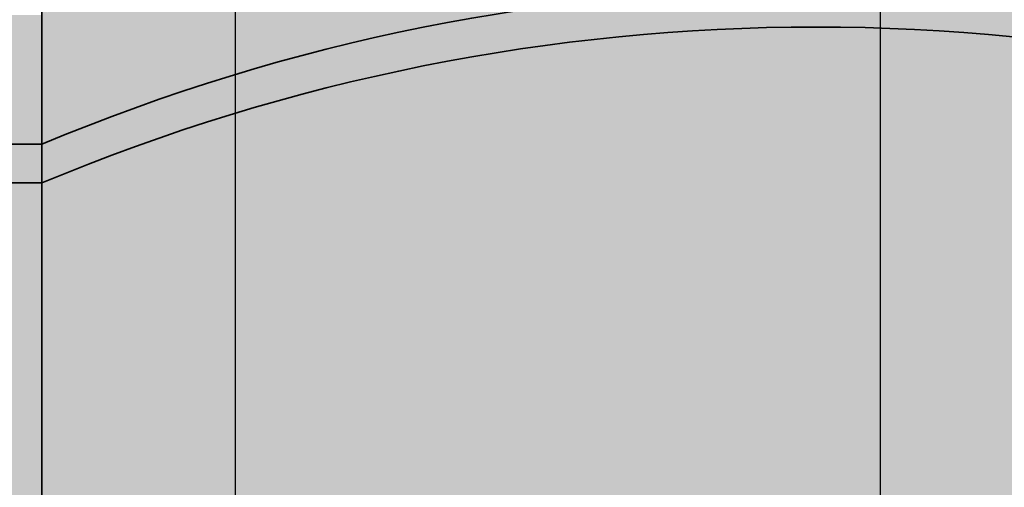
# Model space of a CAD drawing. Units: millimetres. Extents: x 130 to 1021, y 147 to 699.
# Tile 19 of 40: x 366 to 442, y 440 to 477. Entities that reach past the tile are written whole.
import ezdxf

# ---------------------------------------------------------------- set-up
doc = ezdxf.new("R2010")
doc.units = ezdxf.units.MM
doc.header["$MEASUREMENT"] = 0
for name, color, linetype, lineweight in [('A-ANNO-DIMS', 2, 'Continuous', 18), ('A-ELEV', 7, 'Continuous', 35), ('A-ELEV-PATT', 9, 'Continuous', 13)]:
    doc.layers.add(name, color=color, linetype=linetype, lineweight=lineweight)
doc.styles.get("Standard").update_dxf_attribs({"font": 'arial.ttf'})
doc.dimstyles.get("Standard").update_dxf_attribs({"dimtxt": 20, "dimasz": 10, "dimexe": 10, "dimexo": 10, "dimgap": 5, "dimtad": 0, "dimtih": 1, "dimtoh": 1, "dimdec": 0, "dimzin": 0, "dimdsep": 46, "dimtxsty": 'Standard', "dimcen": 5, "dimadec": 0, "dimazin": 0, "dimtfac": 1, "dimtdec": 0, "dimtofl": 0, "dimtmove": 0, "dimatfit": 3, "dimfxl": 1, "dimtolj": 1, "dimtzin": 0, "dimarcsym": 0})

# ---------------------------------------------------------------- blocks, each defined once
blk = doc.blocks.new('*D11')
at = {"layer": 'A-ANNO-DIMS', "color": 0, "lineweight": -2, "transparency": 16777216}
for p, q in [((737.374, 648.699), (737.374, 149.739)), ((299.374, 566.947), (299.374, 149.739)), ((309.374, 159.739), (490.857, 159.739)), ((727.374, 159.739), (545.891, 159.739))]:
    blk.add_line(p, q, dxfattribs=at)
at = {"layer": 'A-ANNO-DIMS', "color": 0, "transparency": 16777216}
for points in [[(309.374, 161.406), (309.374, 158.073), (299.374, 159.739)], [(727.374, 161.406), (727.374, 158.073), (737.374, 159.739)]]:
    blk.add_solid(points, dxfattribs=at)
at = {"layer": 'Defpoints', "color": 0, "transparency": 16777216}
for p in [(737.374, 658.699), (299.374, 576.947), (737.374, 159.739)]:
    blk.add_point(p, dxfattribs=at)
at = {"layer": 'A-ANNO-DIMS', "color": 0, "transparency": 16777216, "insert": (518.374, 159.739), "char_height": 20, "attachment_point": 5}
blk.add_mtext('\\A1;438', dxfattribs=at)
blk = doc.blocks.new('*D12')
at = {"layer": 'A-ANNO-DIMS', "color": 0, "lineweight": -2, "transparency": 16777216}
for p, q in [((477.374, 661.947), (265.074, 661.947)), ((275.074, 651.947), (275.074, 438.205)), ((275.074, 194.039), (275.074, 407.782)), ((357.163, 184.039), (265.074, 184.039))]:
    blk.add_line(p, q, dxfattribs=at)
at = {"layer": 'A-ANNO-DIMS', "color": 0, "transparency": 16777216}
for points in [[(273.407, 651.947), (276.74, 651.947), (275.074, 661.947)], [(273.407, 194.039), (276.74, 194.039), (275.074, 184.039)]]:
    blk.add_solid(points, dxfattribs=at)
at = {"layer": 'Defpoints', "color": 0, "transparency": 16777216}
for p in [(275.074, 661.947), (487.374, 661.947), (367.163, 184.039)]:
    blk.add_point(p, dxfattribs=at)
at = {"layer": 'A-ANNO-DIMS', "color": 0, "transparency": 16777216, "insert": (275.074, 422.993), "char_height": 20, "attachment_point": 5}
blk.add_mtext('\\A1;477.9', dxfattribs=at)
blk = doc.blocks.new('*D15')
at = {"layer": 'A-ANNO-DIMS', "color": 0, "lineweight": -2, "transparency": 16777216}
for p, q in [((327.374, 579.884), (327.374, 696.247)), ((357.941, 411.947), (357.941, 696.247)), ((337.374, 686.247), (347.941, 686.247)), ((357.941, 686.247), (367.941, 686.247))]:
    blk.add_line(p, q, dxfattribs=at)
at = {"layer": 'A-ANNO-DIMS', "color": 0, "transparency": 16777216}
for points in [[(337.374, 687.914), (337.374, 684.581), (327.374, 686.247)], [(347.941, 687.914), (347.941, 684.581), (357.941, 686.247)]]:
    blk.add_solid(points, dxfattribs=at)
at = {"layer": 'Defpoints', "color": 0, "transparency": 16777216}
for p in [(357.941, 686.247), (327.374, 569.884), (357.941, 401.947)]:
    blk.add_point(p, dxfattribs=at)
at = {"layer": 'A-ANNO-DIMS', "color": 0, "transparency": 16777216, "insert": (406.679, 686.247), "char_height": 20, "attachment_point": 5}
blk.add_mtext('\\A1;30.57', dxfattribs=at)
blk = doc.blocks.new('*D16')
at = {"layer": 'A-ANNO-DIMS', "color": 0, "lineweight": -2, "transparency": 16777216}
for p, q in [((357.941, 411.947), (357.941, 696.247)), ((363.922, 579.884), (363.922, 696.247)), ((347.941, 686.247), (337.941, 686.247)), ((373.922, 686.247), (383.922, 686.247))]:
    blk.add_line(p, q, dxfattribs=at)
at = {"layer": 'A-ANNO-DIMS', "color": 0, "transparency": 16777216}
for points in [[(347.941, 687.914), (347.941, 684.581), (357.941, 686.247)], [(373.922, 687.914), (373.922, 684.581), (363.922, 686.247)]]:
    blk.add_solid(points, dxfattribs=at)
at = {"layer": 'Defpoints', "color": 0, "transparency": 16777216}
for p in [(363.922, 686.247), (363.922, 569.884), (357.941, 401.947)]:
    blk.add_point(p, dxfattribs=at)
at = {"layer": 'A-ANNO-DIMS', "color": 0, "transparency": 16777216, "insert": (420.737, 686.247), "char_height": 20, "attachment_point": 5}
blk.add_mtext('\\A1;5.981', dxfattribs=at)
blk = doc.blocks.new('*D18')
at = {"layer": 'A-ANNO-DIMS', "color": 0, "lineweight": -2, "transparency": 16777216}
for p, q in [((375.85, 490.216), (375.85, 696.247)), ((382.374, 388.947), (382.374, 696.247)), ((365.85, 686.247), (355.85, 686.247)), ((392.374, 686.247), (402.374, 686.247))]:
    blk.add_line(p, q, dxfattribs=at)
at = {"layer": 'A-ANNO-DIMS', "color": 0, "transparency": 16777216}
for points in [[(365.85, 687.914), (365.85, 684.581), (375.85, 686.247)], [(392.374, 687.914), (392.374, 684.581), (382.374, 686.247)]]:
    blk.add_solid(points, dxfattribs=at)
at = {"layer": 'Defpoints', "color": 0, "transparency": 16777216}
for p in [(382.374, 686.247), (375.85, 480.216), (382.374, 378.947)]:
    blk.add_point(p, dxfattribs=at)
at = {"layer": 'A-ANNO-DIMS', "color": 0, "transparency": 16777216, "insert": (441.132, 686.247), "char_height": 20, "attachment_point": 5}
blk.add_mtext('\\A1;6.524', dxfattribs=at)
blk = doc.blocks.new('*D19')
at = {"layer": 'A-ANNO-DIMS', "color": 0, "lineweight": -2, "transparency": 16777216}
for p, q in [((382.374, 388.947), (382.374, 696.247)), ((414.652, 510.881), (414.652, 696.247)), ((392.374, 686.247), (404.652, 686.247)), ((414.652, 686.247), (424.652, 686.247))]:
    blk.add_line(p, q, dxfattribs=at)
at = {"layer": 'A-ANNO-DIMS', "color": 0, "transparency": 16777216}
for points in [[(392.374, 687.914), (392.374, 684.581), (382.374, 686.247)], [(404.652, 687.914), (404.652, 684.581), (414.652, 686.247)]]:
    blk.add_solid(points, dxfattribs=at)
at = {"layer": 'Defpoints', "color": 0, "transparency": 16777216}
for p in [(414.652, 686.247), (414.652, 500.881), (382.374, 378.947)]:
    blk.add_point(p, dxfattribs=at)
at = {"layer": 'A-ANNO-DIMS', "color": 0, "transparency": 16777216, "insert": (463.411, 686.247), "char_height": 20, "attachment_point": 5}
blk.add_mtext('\\A1;32.28', dxfattribs=at)
blk = doc.blocks.new('*D20')
at = {"layer": 'A-ANNO-DIMS', "color": 0, "lineweight": -2, "transparency": 16777216}
for p, q in [((414.652, 510.881), (414.652, 696.247)), ((432.374, 388.947), (432.374, 696.247)), ((404.652, 686.247), (394.652, 686.247)), ((442.374, 686.247), (452.374, 686.247))]:
    blk.add_line(p, q, dxfattribs=at)
at = {"layer": 'A-ANNO-DIMS', "color": 0, "transparency": 16777216}
for points in [[(404.652, 687.914), (404.652, 684.581), (414.652, 686.247)], [(442.374, 687.914), (442.374, 684.581), (432.374, 686.247)]]:
    blk.add_solid(points, dxfattribs=at)
at = {"layer": 'Defpoints', "color": 0, "transparency": 16777216}
for p in [(432.374, 686.247), (414.652, 500.881), (432.374, 378.947)]:
    blk.add_point(p, dxfattribs=at)
at = {"layer": 'A-ANNO-DIMS', "color": 0, "transparency": 16777216, "insert": (490.075, 686.247), "char_height": 20, "attachment_point": 5}
blk.add_mtext('\\A1;17.72', dxfattribs=at)
blk = doc.blocks.new('*D21')
at = {"layer": 'A-ANNO-DIMS', "color": 0, "lineweight": -2, "transparency": 16777216}
for p, q in [((432.374, 388.947), (432.374, 696.247)), ((447.374, 656.947), (447.374, 696.247)), ((422.374, 686.247), (412.374, 686.247)), ((457.374, 686.247), (467.374, 686.247))]:
    blk.add_line(p, q, dxfattribs=at)
at = {"layer": 'A-ANNO-DIMS', "color": 0, "transparency": 16777216}
for points in [[(422.374, 687.914), (422.374, 684.581), (432.374, 686.247)], [(457.374, 687.914), (457.374, 684.581), (447.374, 686.247)]]:
    blk.add_solid(points, dxfattribs=at)
at = {"layer": 'Defpoints', "color": 0, "transparency": 16777216}
for p in [(447.374, 686.247), (447.374, 646.947), (432.374, 378.947)]:
    blk.add_point(p, dxfattribs=at)
at = {"layer": 'A-ANNO-DIMS', "color": 0, "transparency": 16777216, "insert": (485.832, 686.247), "char_height": 20, "attachment_point": 5}
blk.add_mtext('\\A1;15', dxfattribs=at)
blk = doc.blocks.new('*D22')
at = {"layer": 'A-ANNO-DIMS', "color": 0, "lineweight": -2, "transparency": 16777216}
for p, q in [((447.374, 656.947), (447.374, 696.247)), ((466.767, 403.947), (466.767, 696.247)), ((437.374, 686.247), (427.374, 686.247)), ((476.767, 686.247), (486.767, 686.247))]:
    blk.add_line(p, q, dxfattribs=at)
at = {"layer": 'A-ANNO-DIMS', "color": 0, "transparency": 16777216}
for points in [[(437.374, 687.914), (437.374, 684.581), (447.374, 686.247)], [(476.767, 687.914), (476.767, 684.581), (466.767, 686.247)]]:
    blk.add_solid(points, dxfattribs=at)
at = {"layer": 'Defpoints', "color": 0, "transparency": 16777216}
for p in [(466.767, 686.247), (447.374, 646.947), (466.767, 393.947)]:
    blk.add_point(p, dxfattribs=at)
at = {"layer": 'A-ANNO-DIMS', "color": 0, "transparency": 16777216, "insert": (532.34, 686.247), "char_height": 20, "attachment_point": 5}
blk.add_mtext('\\A1;19.393', dxfattribs=at)
blk = doc.blocks.new('*D43')
at = {"layer": 'A-ANNO-DIMS', "color": 0, "lineweight": -2, "transparency": 16777216}
for p, q in [((275.074, 510.881), (275.074, 520.881)), ((275.074, 520.881), (285.074, 520.881)), ((404.652, 500.881), (265.074, 500.881)), ((317.374, 480.95), (265.074, 480.95)), ((275.074, 470.95), (275.074, 460.95))]:
    blk.add_line(p, q, dxfattribs=at)
at = {"layer": 'A-ANNO-DIMS', "color": 0, "transparency": 16777216}
for points in [[(273.407, 510.881), (276.74, 510.881), (275.074, 500.881)], [(273.407, 470.95), (276.74, 470.95), (275.074, 480.95)]]:
    blk.add_solid(points, dxfattribs=at)
at = {"layer": 'Defpoints', "color": 0, "transparency": 16777216}
for p in [(275.074, 500.881), (414.652, 500.881), (327.374, 480.95)]:
    blk.add_point(p, dxfattribs=at)
at = {"layer": 'A-ANNO-DIMS', "color": 0, "transparency": 16777216, "insert": (322.877, 520.881), "char_height": 20, "attachment_point": 5}
blk.add_mtext('\\A1;19.93', dxfattribs=at)
blk = doc.blocks.new('*D64')
at = {"layer": 'A-ANNO-DIMS', "color": 0, "lineweight": -2, "transparency": 16777216}
for p, q in [((502.049, 450.926), (502.049, 460.926)), ((497.049, 455.926), (507.049, 455.926)), ((363.96, 263.061), (409.922, 327.255)), ((353.96, 263.061), (363.96, 263.061))]:
    blk.add_line(p, q, dxfattribs=at)
at = {"layer": 'A-ANNO-DIMS', "color": 0, "transparency": 16777216}
blk.add_solid([(408.567, 328.225), (411.277, 326.284), (415.743, 335.385)], dxfattribs=at)
at = {"layer": 'Defpoints', "color": 0, "transparency": 16777216}
for p in [(502.049, 455.926), (415.743, 335.385)]:
    blk.add_point(p, dxfattribs=at)
at = {"layer": 'A-ANNO-DIMS', "color": 0, "transparency": 16777216, "insert": (297.8, 263.061), "char_height": 20, "attachment_point": 5}
blk.add_mtext('\\A1;R148.25', dxfattribs=at)
blk = doc.blocks.new('*D65')
at = {"layer": 'A-ANNO-DIMS', "color": 0, "lineweight": -2, "transparency": 16777216}
for p, q in [((495.463, 509.127), (472.508, 423.108)), ((505.463, 509.127), (495.463, 509.127)), ((427.374, 248.979), (427.374, 258.979)), ((422.374, 253.979), (432.374, 253.979))]:
    blk.add_line(p, q, dxfattribs=at)
at = {"layer": 'A-ANNO-DIMS', "color": 0, "transparency": 16777216}
blk.add_solid([(470.898, 423.538), (474.118, 422.679), (469.93, 413.447)], dxfattribs=at)
at = {"layer": 'Defpoints', "color": 0, "transparency": 16777216}
for p in [(469.93, 413.447), (427.374, 253.979)]:
    blk.add_point(p, dxfattribs=at)
at = {"layer": 'A-ANNO-DIMS', "color": 0, "transparency": 16777216, "insert": (561.623, 509.127), "char_height": 20, "attachment_point": 5}
blk.add_mtext('\\A1;R165.05', dxfattribs=at)
blk = doc.blocks.new('*D66')
at = {"layer": 'A-ANNO-DIMS', "color": 0, "lineweight": -2, "transparency": 16777216}
for p, q in [((341.579, 557.194), (351.579, 557.194)), ((351.579, 557.194), (376.947, 478.135)), ((427.374, 315.978), (427.374, 325.978)), ((422.374, 320.978), (432.374, 320.978))]:
    blk.add_line(p, q, dxfattribs=at)
at = {"layer": 'A-ANNO-DIMS', "color": 0, "transparency": 16777216}
blk.add_solid([(378.534, 478.644), (375.36, 477.626), (380.002, 468.613)], dxfattribs=at)
at = {"layer": 'Defpoints', "color": 0, "transparency": 16777216}
for p in [(380.002, 468.613), (427.374, 320.978)]:
    blk.add_point(p, dxfattribs=at)
at = {"layer": 'A-ANNO-DIMS', "color": 0, "transparency": 16777216, "insert": (263.53, 557.194), "char_height": 20, "attachment_point": 5}
blk.add_mtext('\\A1;4X R155.05', dxfattribs=at)
blk = doc.blocks.new('*D67')
at = {"layer": 'A-ANNO-DIMS', "color": 0, "lineweight": -2, "transparency": 16777216}
for p, q in [((479.756, 492.431), (462.144, 412.223)), ((489.756, 492.431), (479.756, 492.431)), ((427.07, 247.496), (427.07, 257.496)), ((422.07, 252.496), (432.07, 252.496))]:
    blk.add_line(p, q, dxfattribs=at)
at = {"layer": 'A-ANNO-DIMS', "color": 0, "transparency": 16777216}
blk.add_solid([(460.516, 412.58), (463.772, 411.865), (459.999, 402.455)], dxfattribs=at)
at = {"layer": 'Defpoints', "color": 0, "transparency": 16777216}
for p in [(459.999, 402.455), (427.07, 252.496)]:
    blk.add_point(p, dxfattribs=at)
at = {"layer": 'A-ANNO-DIMS', "color": 0, "transparency": 16777216, "insert": (545.841, 492.431), "char_height": 20, "attachment_point": 5}
blk.add_mtext('\\A1;R153.53', dxfattribs=at)
blk = doc.blocks.new('*D68')
at = {"layer": 'A-ANNO-DIMS', "color": 0, "lineweight": -2, "transparency": 16777216}
for p, q in [((361.841, 579.756), (371.841, 579.756)), ((371.841, 579.756), (392.167, 506.693)), ((433.191, 354.23), (433.191, 364.23)), ((428.191, 359.23), (438.191, 359.23))]:
    blk.add_line(p, q, dxfattribs=at)
at = {"layer": 'A-ANNO-DIMS', "color": 0, "transparency": 16777216}
blk.add_solid([(393.773, 507.14), (390.561, 506.246), (394.847, 497.059)], dxfattribs=at)
at = {"layer": 'Defpoints', "color": 0, "transparency": 16777216}
for p in [(394.847, 497.059), (433.191, 359.23)]:
    blk.add_point(p, dxfattribs=at)
at = {"layer": 'A-ANNO-DIMS', "color": 0, "transparency": 16777216, "insert": (305.764, 579.756), "char_height": 20, "attachment_point": 5}
blk.add_mtext('\\A1;R143.06', dxfattribs=at)
blk = doc.blocks.new('*D69')
at = {"layer": 'A-ANNO-DIMS', "color": 0, "lineweight": -2, "transparency": 16777216}
for p, q in [((507.746, 572.261), (483.091, 501.813)), ((517.746, 572.261), (507.746, 572.261)), ((433.191, 354.23), (433.191, 364.23)), ((428.191, 359.23), (438.191, 359.23))]:
    blk.add_line(p, q, dxfattribs=at)
at = {"layer": 'A-ANNO-DIMS', "color": 0, "transparency": 16777216}
blk.add_solid([(481.518, 502.363), (484.664, 501.262), (479.788, 492.374)], dxfattribs=at)
at = {"layer": 'Defpoints', "color": 0, "transparency": 16777216}
for p in [(479.788, 492.374), (433.191, 359.23)]:
    blk.add_point(p, dxfattribs=at)
at = {"layer": 'A-ANNO-DIMS', "color": 0, "transparency": 16777216, "insert": (573.824, 572.261), "char_height": 20, "attachment_point": 5}
blk.add_mtext('\\A1;R141.06', dxfattribs=at)
blk = doc.blocks.new('*D70')
at = {"layer": 'A-ANNO-DIMS', "color": 0, "lineweight": -2, "transparency": 16777216}
for p, q in [((370.141, 588.4), (380.141, 588.4)), ((380.141, 588.4), (397.473, 517.008)), ((432.65, 367.109), (432.65, 377.109)), ((427.65, 372.109), (437.65, 372.109))]:
    blk.add_line(p, q, dxfattribs=at)
at = {"layer": 'A-ANNO-DIMS', "color": 0, "transparency": 16777216}
blk.add_solid([(399.093, 517.402), (395.854, 516.615), (399.832, 507.291)], dxfattribs=at)
at = {"layer": 'Defpoints', "color": 0, "transparency": 16777216}
for p in [(399.832, 507.291), (432.65, 372.109)]:
    blk.add_point(p, dxfattribs=at)
at = {"layer": 'A-ANNO-DIMS', "color": 0, "transparency": 16777216, "insert": (323.757, 588.4), "char_height": 20, "attachment_point": 5}
blk.add_mtext('\\A1;R139.1', dxfattribs=at)
blk = doc.blocks.new('*D71')
at = {"layer": 'A-ANNO-DIMS', "color": 0, "lineweight": -2, "transparency": 16777216}
for p, q in [((492.108, 581.609), (472.542, 512.666)), ((502.108, 581.609), (492.108, 581.609)), ((432.65, 367.109), (432.65, 377.109)), ((427.65, 372.109), (437.65, 372.109))]:
    blk.add_line(p, q, dxfattribs=at)
at = {"layer": 'A-ANNO-DIMS', "color": 0, "transparency": 16777216}
blk.add_solid([(470.938, 513.121), (474.145, 512.211), (469.812, 503.046)], dxfattribs=at)
at = {"layer": 'Defpoints', "color": 0, "transparency": 16777216}
for p in [(469.812, 503.046), (432.65, 372.109)]:
    blk.add_point(p, dxfattribs=at)
at = {"layer": 'A-ANNO-DIMS', "color": 0, "transparency": 16777216, "insert": (548.493, 581.609), "char_height": 20, "attachment_point": 5}
blk.add_mtext('\\A1;R136.1', dxfattribs=at)
blk = doc.blocks.new('*D72')
at = {"layer": 'A-ANNO-DIMS', "color": 0, "lineweight": -2, "transparency": 16777216}
for p, q in [((460.658, 573.64), (451.279, 503.49)), ((470.658, 573.64), (460.658, 573.64)), ((432.115, 355.142), (432.115, 365.142)), ((427.115, 360.142), (437.115, 360.142))]:
    blk.add_line(p, q, dxfattribs=at)
at = {"layer": 'A-ANNO-DIMS', "color": 0, "transparency": 16777216}
blk.add_solid([(449.628, 503.711), (452.931, 503.27), (449.954, 493.579)], dxfattribs=at)
at = {"layer": 'Defpoints', "color": 0, "transparency": 16777216}
for p in [(449.954, 493.579), (432.115, 360.142)]:
    blk.add_point(p, dxfattribs=at)
at = {"layer": 'A-ANNO-DIMS', "color": 0, "transparency": 16777216, "insert": (526.64, 573.64), "char_height": 20, "attachment_point": 5}
blk.add_mtext('\\A1;R134.62', dxfattribs=at)
blk = doc.blocks.new('*D73')
at = {"layer": 'A-ANNO-DIMS', "color": 0, "lineweight": -2, "transparency": 16777216}
for p, q in [((402.678, 571.448), (412.678, 571.448)), ((412.678, 571.448), (419.051, 502.166)), ((432.115, 355.142), (432.115, 365.142)), ((427.115, 360.142), (437.115, 360.142))]:
    blk.add_line(p, q, dxfattribs=at)
at = {"layer": 'A-ANNO-DIMS', "color": 0, "transparency": 16777216}
blk.add_solid([(420.711, 502.319), (417.391, 502.014), (419.967, 492.208)], dxfattribs=at)
at = {"layer": 'Defpoints', "color": 0, "transparency": 16777216}
for p in [(419.967, 492.208), (432.115, 360.142)]:
    blk.add_point(p, dxfattribs=at)
at = {"layer": 'A-ANNO-DIMS', "color": 0, "transparency": 16777216, "insert": (346.696, 571.448), "char_height": 20, "attachment_point": 5}
blk.add_mtext('\\A1;R132.62', dxfattribs=at)

msp = doc.modelspace()

# ---------------------------------------------------------------- hatches: boundary and pattern name
at = {"layer": 'A-ELEV-PATT'}
h = msp.add_hatch(color=256, dxfattribs=at)
h.dxf.hatch_style = 1
h.paths.add_polyline_path([(737.3738, 658.6988, 0.0135961), (632.4019, 661.9473), (607.3738, 661.9473), (487.3738, 661.9473), (487.3738, 649.9473), (607.3738, 649.9473), (632.3794, 649.9473, -0.0136841), (737.3738, 646.6784)])
h.paths.add_polyline_path([(732.3738, 643.9599, 0.0130529), (632.3738, 646.9473), (607.3738, 646.9473), (487.3738, 646.9473), (487.3738, 596.9473), (632.3738, 596.9473, -0.0130529), (732.3738, 593.9599)])
h.paths.add_polyline_path([(737.3738, 593.6732, 0.0137063), (632.3738, 596.9473), (487.3738, 596.9473), (487.3738, 586.9473), (632.355, 586.9473, -0.0137808), (737.3738, 583.6559)])
h.paths.add_polyline_path([(447.3738, 646.9473), (307.3738, 646.9473), (302.3738, 646.9473), (302.3738, 634.9473), (447.3738, 634.9473)])
h.paths.add_polyline_path([(447.3738, 631.9473), (307.3738, 631.9473), (307.3738, 586.9473), (447.3738, 586.9473)])
h.paths.add_polyline_path([(447.3738, 586.9473), (307.3738, 586.9473), (302.3738, 586.9473), (302.3738, 576.9473), (447.3738, 576.9473)])
h.paths.add_polyline_path([(447.3738, 573.9473), (367.3738, 573.9473), (367.3738, 539.9473), (447.3738, 539.9473)])
h.paths.add_polyline_path([(447.3738, 537.9473), (367.3738, 537.9473), (367.3738, 507.9473), (400.392, 507.4253, -0.001728), (401.3281, 507.6451, -0.5220025), (425.6117, 511.0391, -0.0391849), (447.3738, 510.4359), (447.3738, 510.7883)])
h.paths.add_polyline_path([(394.7238, 505.9473), (367.3738, 505.9473), (367.3738, 476.9473, -0.0146512), (375.8501, 480.2159), (376.1506, 499.2266, -0.0355419)])
h.paths.add_polyline_path([(632.3738, 583.9473), (552.3738, 583.9473), (552.3738, 550.9473), (632.3738, 550.9473)])
h.paths.add_polyline_path([(632.3738, 548.9473), (552.3738, 548.9473), (552.3738, 515.9473), (632.3738, 515.9473)])
h.paths.add_polyline_path([(632.3738, 513.9473), (552.3738, 513.9473), (552.3738, 476.9473), (632.3738, 476.9473)])
h.paths.add_polyline_path([(737.3738, 473.6903, 0.0136326), (632.3926, 476.9473), (552.3738, 476.9473), (487.3738, 476.9473), (487.3738, 466.9473), (632.3738, 466.9473, -0.0137063), (737.3738, 463.6732)])
h.paths.add_polyline_path([(732.3738, 460.9552, 0.0130741), (632.3681, 463.9473), (487.3738, 463.9473), (487.3738, 407.735, -0.0032286), (489.3544, 406.9473), (632.3926, 406.9473, -0.0129826), (732.3738, 403.9755)])
h.paths.add_polyline_path([(487.3738, 463.9473, 0.20133), (367.3738, 463.9473), (367.3738, 407.735, -0.1882031), (487.3738, 407.735)])
h.paths.add_polyline_path([(367.3738, 476.9473), (367.3738, 466.9473, -0.2013309), (487.3738, 466.9473), (487.3738, 476.9473, 0.20133)])
h.paths.add_polyline_path([(367.3738, 463.9473), (307.3738, 463.9473), (307.3738, 401.9473), (357.9413, 401.9473), (367.3738, 407.735)])
h.paths.add_polyline_path([(367.3738, 476.9473), (302.3738, 476.9473), (302.3738, 466.9473), (367.3738, 466.9473)])
h.paths.add_polyline_path([(632.8184, 366.9453), (552.3738, 366.9453), (552.3738, 393.9473), (632.8184, 393.9473)])
h.paths.add_polyline_path([(632.8184, 357.2114), (632.8184, 363.9453), (552.3738, 363.9453), (552.3738, 357.2114), (552.3738, 336.9453), (632.8184, 336.9453)])
h.paths.add_polyline_path([(632.8184, 333.9453), (552.3738, 333.9453), (552.3738, 306.9453), (632.8184, 306.9453)])
h.paths.add_polyline_path([(632.8184, 303.9453), (552.3738, 303.9453), (552.3738, 273.9473), (632.355, 273.9473, 0.0000608), (632.8184, 273.9491)])
h.paths.add_polyline_path([(737.3738, 403.6903, 0.0136326), (632.3926, 406.9473), (489.3544, 406.9473, 0.1915481), (367.3738, 407.735), (367.3738, 396.9473, -0.2013309), (487.3738, 396.9473), (632.3738, 396.9473, -0.0137063), (737.3738, 393.6732)])
h.paths.add_polyline_path([(357.9413, 401.9473), (307.3738, 401.9473), (307.3738, 391.9473), (357.9413, 391.9473)])
h.paths.add_polyline_path([(357.9413, 357.2114), (357.9413, 388.9473), (307.3738, 388.9473), (307.3738, 357.2114), (307.3738, 273.9473), (357.9413, 273.9473)])
h.paths.add_polyline_path([(732.3738, 263.93, -0.0130317), (632.3794, 260.9473), (466.7667, 260.9473), (466.7667, 240.9473), (469.8406, 236.978), (469.8406, 221.978), (472.9145, 218.0087), (472.9145, 213.9473), (607.3738, 213.9473), (732.3738, 213.9473)])
h.paths.add_polyline_path([(732.3738, 290.889), (722.479, 290.889), (722.479, 301.889), (732.3738, 301.889), (732.3738, 305.889), (722.479, 305.889), (722.479, 316.889), (732.3738, 316.889), (732.3738, 320.889), (722.479, 320.889), (722.479, 331.889), (732.3738, 331.889), (732.3738, 335.889), (722.479, 335.889), (722.479, 346.889), (732.3738, 346.889), (732.3738, 350.889), (722.479, 350.889), (722.479, 361.889), (732.3738, 361.889), (732.3738, 365.889), (722.479, 365.889), (722.479, 376.889), (732.3738, 376.889), (732.3738, 380.889), (722.479, 380.889), (722.479, 391.4848, 0.0005233), (718.479, 391.6843), (718.479, 380.889), (707.479, 380.889), (707.479, 392.1896, 0.0005231), (703.479, 392.3576), (703.479, 380.889), (692.479, 380.889), (692.479, 392.7765, 0.0005229), (688.479, 392.9131), (688.479, 380.889), (677.479, 380.889), (677.479, 393.2456, 0.0005228), (673.479, 393.3508), (673.479, 380.889), (662.479, 380.889), (662.479, 393.597, 0.0005227), (658.479, 393.6709), (658.479, 380.889), (647.479, 380.889), (647.479, 393.8308, 0.0005226), (643.479, 393.8732), (643.479, 380.889), (632.8184, 380.889), (632.8184, 376.889), (643.479, 376.889), (643.479, 365.889), (632.8184, 365.889), (632.8184, 361.889), (643.479, 361.889), (643.479, 350.889), (632.8184, 350.889), (632.8184, 346.889), (643.479, 346.889), (643.479, 335.889), (632.8184, 335.889), (632.8184, 331.889), (643.479, 331.889), (643.479, 320.889), (632.8184, 320.889), (632.8184, 316.889), (643.479, 316.889), (643.479, 305.889), (632.8184, 305.889), (632.8184, 301.889), (643.479, 301.889), (643.479, 290.889), (632.8184, 290.889), (632.8184, 286.889), (643.479, 286.889), (643.479, 274.0217, 0.0005246), (647.479, 274.0643), (647.479, 286.889), (658.479, 286.889), (658.479, 274.2248, 0.0005246), (662.479, 274.2989), (662.479, 286.889), (673.479, 286.889), (673.479, 274.546, 0.0005247), (677.479, 274.6516), (677.479, 286.889), (688.479, 286.889), (688.479, 274.9853, 0.0005248), (692.479, 275.1224), (692.479, 286.889), (703.479, 286.889), (703.479, 275.5429, 0.000525), (707.479, 275.7115), (707.479, 286.889), (718.479, 286.889), (718.479, 276.2187, 0.0005252), (722.479, 276.4189), (722.479, 286.889), (732.3738, 286.889)])
h.paths.add_polyline_path([(718.479, 290.889), (707.479, 290.889), (707.479, 301.889), (718.479, 301.889)], flags=16)
h.paths.add_polyline_path([(703.479, 290.889), (692.479, 290.889), (692.479, 301.889), (703.479, 301.889)], flags=16)
h.paths.add_polyline_path([(718.479, 305.889), (707.479, 305.889), (707.479, 316.889), (718.479, 316.889)], flags=16)
h.paths.add_polyline_path([(703.479, 305.889), (692.479, 305.889), (692.479, 316.889), (703.479, 316.889)], flags=16)
h.paths.add_polyline_path([(688.479, 290.889), (677.479, 290.889), (677.479, 301.889), (688.479, 301.889)], flags=16)
h.paths.add_polyline_path([(718.479, 320.889), (707.479, 320.889), (707.479, 331.889), (718.479, 331.889)], flags=16)
h.paths.add_polyline_path([(688.479, 305.889), (677.479, 305.889), (677.479, 316.889), (688.479, 316.889)], flags=16)
h.paths.add_polyline_path([(703.479, 320.889), (692.479, 320.889), (692.479, 331.889), (703.479, 331.889)], flags=16)
h.paths.add_polyline_path([(688.479, 320.889), (677.479, 320.889), (677.479, 331.889), (688.479, 331.889)], flags=16)
h.paths.add_polyline_path([(673.479, 290.889), (662.479, 290.889), (662.479, 301.889), (673.479, 301.889)], flags=16)
h.paths.add_polyline_path([(718.479, 335.889), (707.479, 335.889), (707.479, 346.889), (718.479, 346.889)], flags=16)
h.paths.add_polyline_path([(673.479, 305.889), (662.479, 305.889), (662.479, 316.889), (673.479, 316.889)], flags=16)
h.paths.add_polyline_path([(703.479, 335.889), (692.479, 335.889), (692.479, 346.889), (703.479, 346.889)], flags=16)
h.paths.add_polyline_path([(673.479, 320.889), (662.479, 320.889), (662.479, 331.889), (673.479, 331.889)], flags=16)
h.paths.add_polyline_path([(688.479, 335.889), (677.479, 335.889), (677.479, 346.889), (688.479, 346.889)], flags=16)
h.paths.add_polyline_path([(658.479, 290.889), (647.479, 290.889), (647.479, 301.889), (658.479, 301.889)], flags=16)
h.paths.add_polyline_path([(718.479, 350.889), (707.479, 350.889), (707.479, 361.889), (718.479, 361.889)], flags=16)
h.paths.add_polyline_path([(658.479, 305.889), (647.479, 305.889), (647.479, 316.889), (658.479, 316.889)], flags=16)
h.paths.add_polyline_path([(703.479, 350.889), (692.479, 350.889), (692.479, 361.889), (703.479, 361.889)], flags=16)
h.paths.add_polyline_path([(673.479, 335.889), (662.479, 335.889), (662.479, 346.889), (673.479, 346.889)], flags=16)
h.paths.add_polyline_path([(658.479, 320.889), (647.479, 320.889), (647.479, 331.889), (658.479, 331.889)], flags=16)
h.paths.add_polyline_path([(688.479, 350.889), (677.479, 350.889), (677.479, 361.889), (688.479, 361.889)], flags=16)
h.paths.add_polyline_path([(718.479, 365.889), (707.479, 365.889), (707.479, 376.889), (718.479, 376.889)], flags=16)
h.paths.add_polyline_path([(658.479, 335.889), (647.479, 335.889), (647.479, 346.889), (658.479, 346.889)], flags=16)
h.paths.add_polyline_path([(673.479, 350.889), (662.479, 350.889), (662.479, 361.889), (673.479, 361.889)], flags=16)
h.paths.add_polyline_path([(703.479, 365.889), (692.479, 365.889), (692.479, 376.889), (703.479, 376.889)], flags=16)
h.paths.add_polyline_path([(688.479, 365.889), (677.479, 365.889), (677.479, 376.889), (688.479, 376.889)], flags=16)
h.paths.add_polyline_path([(658.479, 350.889), (647.479, 350.889), (647.479, 361.889), (658.479, 361.889)], flags=16)
h.paths.add_polyline_path([(673.479, 365.889), (662.479, 365.889), (662.479, 376.889), (673.479, 376.889)], flags=16)
h.paths.add_polyline_path([(658.479, 365.889), (647.479, 365.889), (647.479, 376.889), (658.479, 376.889)], flags=16)
h.paths.add_polyline_path([(732.3738, 503.9786), (722.3392, 503.9786), (722.3392, 514.9786), (732.3738, 514.9786), (732.3738, 518.9786), (722.3392, 518.9786), (722.3392, 529.9786), (732.3738, 529.9786), (732.3738, 533.9786), (722.3392, 533.9786), (722.3392, 544.9786), (732.3738, 544.9786), (732.3738, 546.9473), (732.3738, 548.9786), (722.3392, 548.9786), (722.3392, 559.9786), (732.3738, 559.9786), (732.3738, 563.9786), (722.3392, 563.9786), (722.3392, 574.9786), (732.3738, 574.9786), (732.3738, 578.9786), (722.3392, 578.9786), (722.3392, 581.4789, 0.000526), (718.3392, 581.6791), (718.3392, 578.9786), (707.3392, 578.9786), (707.3392, 582.1863, 0.0005258), (703.3392, 582.355), (703.3392, 578.9786), (692.3392, 578.9786), (692.3392, 582.7752, 0.0005257), (688.3392, 582.9123), (688.3392, 578.9786), (677.3392, 578.9786), (677.3392, 583.2457, 0.0005255), (673.3392, 583.3512), (673.3392, 578.9786), (662.3392, 578.9786), (662.3392, 583.5978, 0.0005254), (658.3392, 583.6718), (658.3392, 578.9786), (647.3392, 578.9786), (647.3392, 583.8317, 0.0005254), (643.3392, 583.8741), (643.3392, 578.9786), (632.3738, 578.9786), (632.3738, 574.9786), (643.3392, 574.9786), (643.3392, 563.9786), (632.3738, 563.9786), (632.3738, 559.9786), (643.3392, 559.9786), (643.3392, 548.9786), (632.3738, 548.9786), (632.3738, 544.9786), (643.3392, 544.9786), (643.3392, 533.9786), (632.3738, 533.9786), (632.3738, 529.9786), (643.3392, 529.9786), (643.3392, 518.9786), (632.3738, 518.9786), (632.3738, 515.9473), (632.3738, 514.9786), (643.3392, 514.9786), (643.3392, 503.9786), (632.3738, 503.9786), (632.3738, 499.9786), (643.3392, 499.9786), (643.3392, 488.9786), (632.3738, 488.9786), (632.3738, 484.9786), (643.3392, 484.9786), (643.3392, 476.8751, -0.0005191), (647.3392, 476.8332), (647.3392, 484.9786), (658.3392, 484.9786), (658.3392, 476.6752, -0.0005192), (662.3392, 476.6022), (662.3392, 484.9786), (673.3392, 484.9786), (673.3392, 476.3585, -0.0005193), (677.3392, 476.2543), (677.3392, 484.9786), (688.3392, 484.9786), (688.3392, 475.9248, -0.0005194), (692.3392, 475.7894), (692.3392, 484.9786), (703.3392, 484.9786), (703.3392, 475.3741, -0.0005195), (707.3392, 475.2075), (707.3392, 484.9786), (718.3392, 484.9786), (718.3392, 474.7064, -0.0005197), (722.3392, 474.5086), (722.3392, 484.9786), (732.3738, 484.9786), (732.3738, 488.9786), (722.3392, 488.9786), (722.3392, 499.9786), (732.3738, 499.9786)])
h.paths.add_polyline_path([(718.3392, 503.9786), (707.3392, 503.9786), (707.3392, 514.9786), (718.3392, 514.9786)], flags=16)
h.paths.add_polyline_path([(718.3392, 499.9786), (718.3392, 488.9786), (707.3392, 488.9786), (707.3392, 499.9786)], flags=16)
h.paths.add_polyline_path([(718.3392, 518.9786), (707.3392, 518.9786), (707.3392, 529.9786), (718.3392, 529.9786)], flags=16)
h.paths.add_polyline_path([(703.3392, 503.9786), (692.3392, 503.9786), (692.3392, 514.9786), (703.3392, 514.9786)], flags=16)
h.paths.add_polyline_path([(703.3392, 499.9786), (703.3392, 488.9786), (692.3392, 488.9786), (692.3392, 499.9786)], flags=16)
h.paths.add_polyline_path([(703.3392, 518.9786), (692.3392, 518.9786), (692.3392, 529.9786), (703.3392, 529.9786)], flags=16)
h.paths.add_polyline_path([(718.3392, 533.9786), (707.3392, 533.9786), (707.3392, 544.9786), (718.3392, 544.9786)], flags=16)
h.paths.add_polyline_path([(688.3392, 503.9786), (677.3392, 503.9786), (677.3392, 514.9786), (688.3392, 514.9786)], flags=16)
h.paths.add_polyline_path([(688.3392, 499.9786), (688.3392, 488.9786), (677.3392, 488.9786), (677.3392, 499.9786)], flags=16)
h.paths.add_polyline_path([(703.3392, 533.9786), (692.3392, 533.9786), (692.3392, 544.9786), (703.3392, 544.9786)], flags=16)
h.paths.add_polyline_path([(688.3392, 518.9786), (677.3392, 518.9786), (677.3392, 529.9786), (688.3392, 529.9786)], flags=16)
h.paths.add_polyline_path([(688.3392, 533.9786), (677.3392, 533.9786), (677.3392, 544.9786), (688.3392, 544.9786)], flags=16)
h.paths.add_polyline_path([(718.3392, 548.9786), (707.3392, 548.9786), (707.3392, 559.9786), (718.3392, 559.9786)], flags=16)
h.paths.add_polyline_path([(673.3392, 503.9786), (662.3392, 503.9786), (662.3392, 514.9786), (673.3392, 514.9786)], flags=16)
h.paths.add_polyline_path([(673.3392, 499.9786), (673.3392, 488.9786), (662.3392, 488.9786), (662.3392, 499.9786)], flags=16)
h.paths.add_polyline_path([(703.3392, 548.9786), (692.3392, 548.9786), (692.3392, 559.9786), (703.3392, 559.9786)], flags=16)
h.paths.add_polyline_path([(673.3392, 518.9786), (662.3392, 518.9786), (662.3392, 529.9786), (673.3392, 529.9786)], flags=16)
h.paths.add_polyline_path([(688.3392, 548.9786), (677.3392, 548.9786), (677.3392, 559.9786), (688.3392, 559.9786)], flags=16)
h.paths.add_polyline_path([(673.3392, 533.9786), (662.3392, 533.9786), (662.3392, 544.9786), (673.3392, 544.9786)], flags=16)
h.paths.add_polyline_path([(718.3392, 563.9786), (707.3392, 563.9786), (707.3392, 574.9786), (718.3392, 574.9786)], flags=16)
h.paths.add_polyline_path([(658.3392, 503.9786), (647.3392, 503.9786), (647.3392, 514.9786), (658.3392, 514.9786)], flags=16)
h.paths.add_polyline_path([(658.3392, 499.9786), (658.3392, 488.9786), (647.3392, 488.9786), (647.3392, 499.9786)], flags=16)
h.paths.add_polyline_path([(703.3392, 563.9786), (692.3392, 563.9786), (692.3392, 574.9786), (703.3392, 574.9786)], flags=16)
h.paths.add_polyline_path([(658.3392, 518.9786), (647.3392, 518.9786), (647.3392, 529.9786), (658.3392, 529.9786)], flags=16)
h.paths.add_polyline_path([(673.3392, 548.9786), (662.3392, 548.9786), (662.3392, 559.9786), (673.3392, 559.9786)], flags=16)
h.paths.add_polyline_path([(688.3392, 563.9786), (677.3392, 563.9786), (677.3392, 574.9786), (688.3392, 574.9786)], flags=16)
h.paths.add_polyline_path([(658.3392, 533.9786), (647.3392, 533.9786), (647.3392, 544.9786), (658.3392, 544.9786)], flags=16)
h.paths.add_polyline_path([(673.3392, 563.9786), (662.3392, 563.9786), (662.3392, 574.9786), (673.3392, 574.9786)], flags=16)
h.paths.add_polyline_path([(658.3392, 548.9786), (647.3392, 548.9786), (647.3392, 559.9786), (658.3392, 559.9786)], flags=16)
h.paths.add_polyline_path([(658.3392, 563.9786), (647.3392, 563.9786), (647.3392, 574.9786), (658.3392, 574.9786)], flags=16)
h = msp.add_hatch(color=256, dxfattribs=at)
h.dxf.hatch_style = 1
h.paths.add_polyline_path([(447.3738, 576.9473), (302.3738, 576.9473), (302.3738, 573.9473), (447.3738, 573.9473)])
h.paths.add_polyline_path([(487.3738, 583.9473), (487.3738, 586.9473), (447.3738, 576.9473), (447.3738, 573.9473)])
h.paths.add_polyline_path([(632.355, 586.9473), (487.3738, 586.9473), (487.3738, 583.9473), (632.3738, 583.9473), (632.3738, 583.9472, -0.0138), (737.3738, 580.6507), (737.3738, 583.6559, 0.0137808)])
h.paths.add_polyline_path([(367.3738, 466.9473), (302.3738, 466.9473), (302.3738, 463.9473), (367.3738, 463.9473)])
h.paths.add_polyline_path([(487.3738, 463.9473), (487.3738, 466.9473, 0.2013309), (367.3738, 466.9473), (367.3738, 463.9473, -0.20133)])
h.paths.add_polyline_path([(632.3738, 466.9473), (487.3738, 466.9473), (487.3738, 463.9473), (632.3681, 463.9473, -0.0137285), (737.3738, 460.6681), (737.3738, 463.6732, 0.0137063)])
h.paths.add_polyline_path([(632.3738, 396.9473), (487.3738, 396.9473, 0.2013309), (367.3738, 396.9473), (367.3738, 393.9473, -0.2023717), (486.7667, 393.9473), (632.3681, 393.9473, -0.0137285), (737.3738, 390.6681), (737.3738, 393.6732, 0.0137063)])
h.paths.add_polyline_path([(357.9413, 391.9473), (307.3738, 391.9473), (307.3738, 388.9473), (357.9413, 388.9473)])
h.paths.add_polyline_path([(367.3738, 393.9473), (367.3738, 396.9473), (357.9413, 391.924), (357.9413, 388.9473), (358.058, 388.9473)])
h.paths.add_polyline_path([(737.3738, 264.2162), (737.3738, 267.2214, -0.0137063), (632.3738, 263.9473), (463.7667, 263.9473), (466.7667, 260.9473), (632.3794, 260.9473, 0.0136841)])
h.paths.add_polyline_path([(463.7667, 263.9473), (447.3738, 263.9473), (450.3738, 260.9473), (466.7667, 260.9473)])
h.paths.add_polyline_path([(447.3738, 263.9473), (432.3738, 263.9473), (432.3738, 260.9473), (450.3738, 260.9473)])
h.paths.add_polyline_path([(382.3738, 263.9473), (357.9413, 263.9473), (357.9413, 260.9473), (382.3738, 260.9473)])
h.paths.add_polyline_path([(357.9413, 263.9473), (307.3738, 263.9473), (307.3738, 260.9473), (357.9413, 260.9473)])

# ---------------------------------------------------------------- linework, layer by layer
at = {"layer": 'A-ELEV'}
for p, q in [((367.3738, 573.9473), (367.3738, 357.2114)), ((367.3738, 466.9473), (302.3738, 466.9473)), ((367.3738, 466.9473), (357.3742, 466.8599)), ((367.3738, 463.9473), (302.3738, 463.9473))]:
    msp.add_line(p, q, dxfattribs=at)
for centre, radius, start, end in [((427.3738, 323.9788), 155.0484, 67.233534, 112.766466), ((427.3738, 320.9781), 155.049, 67.23363, 112.76637)]:
    msp.add_arc(centre, radius, start, end, dxfattribs=at)

# ---------------------------------------------------------------- dimensions: what is measured, and where the dimension line sits
at = {"layer": 'A-ANNO-DIMS'}
for base, p1, p2, override, picture, middle in [((357.9413, 686.2473), (327.3738, 569.884), (357.9413, 401.9473), {"dimdec": 2, "dimlfac": 1, "dimrnd": 0, "dimzin": 0, "dimdsep": 46, "dimlunit": 2}, '*D15', (406.6794, 686.2473)), ((363.922, 686.2473), (357.9413, 401.9473), (363.922, 569.884), {"dimdec": 3, "dimlfac": 1, "dimrnd": 0, "dimzin": 0, "dimdsep": 46, "dimlunit": 2}, '*D16', (420.7365, 686.2473)), ((382.3738, 686.2473), (375.8501, 480.2159), (382.3738, 378.9473), {"dimdec": 3, "dimlfac": 1, "dimrnd": 0, "dimzin": 0, "dimdsep": 46, "dimlunit": 2}, '*D18', (441.1323, 686.2473)), ((414.6525, 686.2473), (382.3738, 378.9473), (414.6525, 500.8811), {"dimdec": 2, "dimlfac": 1, "dimrnd": 0, "dimzin": 0, "dimdsep": 46, "dimlunit": 2}, '*D19', (463.411, 686.2473)), ((432.3738, 686.2473), (414.6525, 500.8811), (432.3738, 378.9473), {"dimdec": 2, "dimlfac": 1, "dimrnd": 0, "dimzin": 0, "dimdsep": 46, "dimlunit": 2}, '*D20', (490.075, 686.2473)), ((447.3738, 686.2473), (432.3738, 378.9473), (447.3738, 646.9473), {"dimdec": 0, "dimlfac": 1, "dimrnd": 0, "dimzin": 0, "dimdsep": 46, "dimlunit": 2}, '*D21', (485.8322, 686.2473)), ((466.7667, 686.2473), (447.3738, 646.9473), (466.7667, 393.9473), {"dimdec": 3, "dimlfac": 1, "dimrnd": 0, "dimzin": 0, "dimdsep": 46, "dimlunit": 2}, '*D22', (532.3397, 686.2473)), ((737.3738, 159.7395), (299.3738, 576.9473), (737.3738, 658.6988), {"dimdec": 0, "dimlfac": 1, "dimrnd": 0, "dimzin": 0, "dimdsep": 46, "dimlunit": 2}, '*D11', (518.3738, 159.7395))]:
    dim = msp.add_linear_dim(base=base, p1=p1, p2=p2, dimstyle='Standard', override=override, dxfattribs=at)
    dim.commit()
    dim.dimension.update_dxf_attribs({"geometry": picture, "text_midpoint": middle})
for base, p1, p2, override, picture, middle in [((275.0738, 661.9473), (367.163, 184.0395), (487.3738, 661.9473), {"dimdec": 1, "dimlfac": 1, "dimrnd": 0, "dimzin": 0, "dimdsep": 46, "dimlunit": 2}, '*D12', (275.0738, 422.9934)), ((275.0738, 500.8811), (327.3738, 480.95), (414.6525, 500.8811), {"dimdec": 2, "dimlfac": 1, "dimrnd": 0, "dimzin": 0, "dimdsep": 46, "dimlunit": 2}, '*D43', (322.8773, 520.8811))]:
    dim = msp.add_linear_dim(base=base, p1=p1, p2=p2, angle=90, dimstyle='Standard', override=override, dxfattribs=at)
    dim.commit()
    dim.dimension.update_dxf_attribs({"geometry": picture, "text_midpoint": middle})
for center, mpoint, override, picture, middle in [((432.6505, 372.1087), (399.8323, 507.2907), {"dimdec": 1, "dimlfac": 1, "dimrnd": 0, "dimzin": 0, "dimdsep": 46, "dimlunit": 2}, '*D70', (323.7567, 588.3999)), ((432.6505, 372.1087), (469.8116, 503.0461), {"dimdec": 1, "dimlfac": 1, "dimrnd": 0, "dimzin": 0, "dimdsep": 46, "dimlunit": 2}, '*D71', (548.493, 581.6085)), ((433.1906, 359.2304), (394.8473, 497.0587), {"dimdec": 2, "dimlfac": 1, "dimrnd": 0, "dimzin": 0, "dimdsep": 46, "dimlunit": 2}, '*D68', (305.7636, 579.7557)), ((432.115, 360.1423), (449.9544, 493.5786), {"dimdec": 2, "dimlfac": 1, "dimrnd": 0, "dimzin": 0, "dimdsep": 46, "dimlunit": 2}, '*D72', (526.6403, 573.6404)), ((433.1906, 359.2304), (479.788, 492.3743), {"dimdec": 2, "dimlfac": 1, "dimrnd": 0, "dimzin": 0, "dimdsep": 46, "dimlunit": 2}, '*D69', (573.8242, 572.2606)), ((432.115, 360.1423), (419.967, 492.2083), {"dimdec": 2, "dimlfac": 1, "dimrnd": 0, "dimzin": 0, "dimdsep": 46, "dimlunit": 2}, '*D73', (346.696, 571.4479)), ((427.3738, 253.9788), (469.9297, 413.4465), {"dimdec": 2, "dimlfac": 1, "dimrnd": 0, "dimzin": 0, "dimdsep": 46, "dimlunit": 2}, '*D65', (561.6228, 509.1272)), ((427.0702, 252.4956), (459.999, 402.4554), {"dimdec": 2, "dimlfac": 1, "dimrnd": 0, "dimzin": 0, "dimdsep": 46, "dimlunit": 2}, '*D67', (545.8408, 492.4313)), ((502.0489, 455.9263), (415.7433, 335.3854), {"dimdec": 2, "dimlfac": 1, "dimrnd": 0, "dimzin": 0, "dimdsep": 46, "dimlunit": 2}, '*D64', (297.8003, 263.0608))]:
    dim = msp.add_radius_dim(center=center, mpoint=mpoint, dimstyle='Standard', override=override, dxfattribs=at)
    dim.commit()
    dim.dimension.update_dxf_attribs({"geometry": picture, "text_midpoint": middle, "dimtype": 164})
dim = msp.add_radius_dim(center=(427.3738, 320.9781), mpoint=(380.0022, 468.6132), text='4X <>', dimstyle='Standard', override={"dimdec": 2, "dimlfac": 1, "dimrnd": 0, "dimzin": 0, "dimdsep": 46, "dimlunit": 2}, dxfattribs=at)
dim.commit()
dim.dimension.update_dxf_attribs({"geometry": '*D66', "text_midpoint": (263.5301, 557.1943), "dimtype": 164})

doc.saveas('drawing.dxf')
